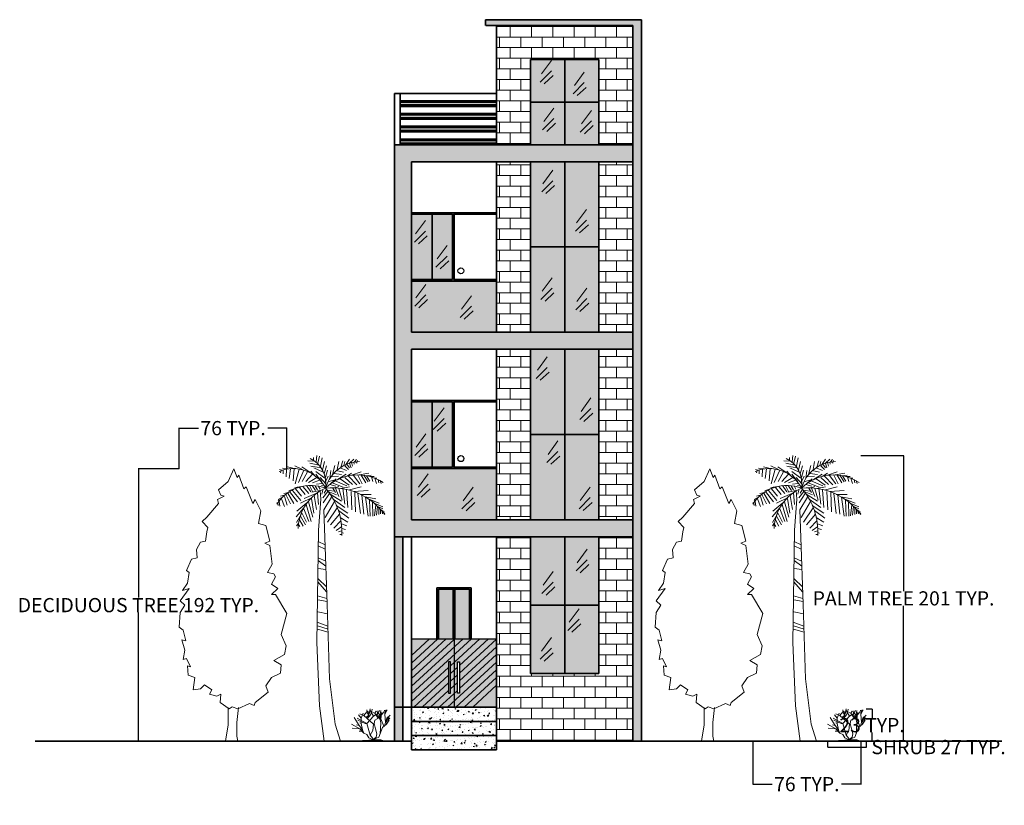
# Model space of a CAD drawing. Units: inches. Extents: x 108 to 802, y 307 to 860.
import ezdxf

# ---------------------------------------------------------------- set-up
doc = ezdxf.new("R2010")
doc.units = ezdxf.units.IN
doc.header["$MEASUREMENT"] = 0
for name, color, linetype, lineweight in [('A-ANNO-DIMS', 2, 'Continuous', 18), ('A-DOOR', 3, 'Continuous', 25), ('A-DOOR-PATT', 18, 'Continuous', 13), ('A-ELEV', 7, 'Continuous', 35), ('A-ELEV-PATT', 251, 'Continuous', 13), ('A-FLOR-STRS', 252, 'Continuous', 13), ('A-GLAZ', 4, 'Continuous', 18), ('A-GLAZ-PATT', 9, 'Continuous', 13), ('A-WALL-PATT', 8, 'Continuous', 13), ('PLANT', 3, 'Continuous', 18)]:
    doc.layers.add(name, color=color, linetype=linetype, lineweight=lineweight)
doc.styles.get("Standard").update_dxf_attribs({"font": 'arial.ttf'})
doc.dimstyles.get("Standard").update_dxf_attribs({"dimtxt": 10, "dimasz": 0.18, "dimexe": 0.18, "dimexo": 0.0625, "dimgap": 0.09, "dimtad": 0, "dimtih": 1, "dimtoh": 1, "dimdec": 0, "dimzin": 0, "dimdsep": 46, "dimlunit": 3, "dimtxsty": 'Standard', "dimcen": 0.09, "dimadec": 0, "dimazin": 0, "dimtfac": 1, "dimtdec": 0, "dimtofl": 0, "dimtmove": 0, "dimatfit": 3, "dimfxl": 1, "dimtolj": 1, "dimtzin": 0, "dimarcsym": 0})

# ---------------------------------------------------------------- blocks, each defined once
blk = doc.blocks.new('Shrub - elevation')
for p, q in [((-12.471, 19.775), (-12.898, 22.044)), ((-11.28, 19.619), (-12.104, 21.184)), ((-11.433, 18.289), (-10.457, 22.749)), ((-8.16, 17.76), (-10.56, 21.6)), ((-9.48, 19.775), (-8.992, 22.592)), ((-7.2, 19.68), (-6.24, 21.12)), ((-5.086, 17.741), (-5.513, 21.34)), ((-5.28, 19.2), (-3.84, 21.6)), ((-3.377, 18.602), (-2.888, 21.575)), ((-0.508, 21.888), (-0.081, 20.558)), ((-0.203, 19.149), (0.102, 21.34)), ((-0.02, 20.01), (0.896, 21.105)), ((0.041, 20.714), (1.384, 22.044)), ((0.102, 21.34), (0.835, 21.888)), ((-18.24, 11.04), (-21.755, 16.655)), ((-12.96, 12.48), (-19.68, 16.32)), ((-13.92, 12.48), (-19.2, 14.88)), ((-16.8, 16.32), (-18.72, 18.72)), ((-14.88, 18.24), (-17.76, 19.2)), ((-16.8, 16.32), (-15.36, 19.68)), ((-16.8, 12.48), (-16.8, 16.32)), ((-14.88, 18.24), (-12.96, 20.64)), ((-8.16, 12), (-14.88, 18.24)), ((-13.325, 16.724), (-11.433, 18.289)), ((-12.96, 12.48), (-8.16, 17.76)), ((-11.677, 19.071), (-12.471, 19.775)), ((-12.043, 15.628), (-11.921, 18.836)), ((-11.982, 16.802), (-10.579, 18.054)), ((-11.921, 18.836), (-10.64, 20.401)), ((-10.579, 18.054), (-9.846, 19.697)), ((-7.2, 19.68), (-8.64, 20.16)), ((-8.16, 17.76), (-5.28, 19.2)), ((-7.68, 12.48), (-7.2, 14.88)), ((-4.8, 16.32), (-7.2, 19.68)), ((-7.2, 14.88), (-3.84, 16.8)), ((-3.377, 15.315), (-5.086, 17.819)), ((-2.88, 12.96), (-4.32, 19.68)), ((-3.84, 16.8), (-0.96, 20.64)), ((-2.766, 16.802), (-3.377, 18.602)), ((-2.88, 15.84), (-2.4, 20.16)), ((-0.96, 10.56), (-2.88, 15.84)), ((0.346, 13.203), (-0.203, 19.149)), ((-0.142, 19.384), (0.59, 20.401)), ((0.346, 13.203), (1.323, 16.254)), ((0.96, 12), (1.44, 15.36)), ((0.96, 12), (2.88, 14.88)), ((1.323, 16.254), (3.642, 18.289)), ((1.44, 15.36), (2.88, 17.28)), ((1.92, 13.44), (2.4, 15.36)), ((2.4, 15.36), (3.36, 16.32)), ((-17.76, 8.64), (-23.663, 11.961)), ((-17.76, 8.64), (-23.128, 9.222)), ((-18.24, 11.04), (-20.16, 11.52)), ((-15.84, 8.16), (-18.24, 11.04)), ((-16.32, 7.2), (-18.24, 7.2)), ((-16.8, 12.48), (-17.76, 12.96)), ((-14.88, 5.76), (-17.76, 8.64)), ((-15.84, 8.16), (-16.8, 12.48)), ((-14.88, 5.76), (-15.84, 8.16)), ((-12.96, 12.48), (-13.92, 12.48)), ((-10.56, 4.32), (-12.96, 12.48)), ((-10.56, 4.32), (-8.64, 7.68)), ((-8.64, 7.68), (-8.16, 12)), ((-6.72, 8.64), (-7.68, 12.48)), ((-5.76, 5.28), (-6.72, 8.64)), ((-4.32, 2.88), (-1.92, 9.6)), ((-3.36, 5.28), (-2.88, 12.96)), ((-1.92, 9.6), (0.96, 12)), ((-0.48, 10.8), (0.346, 13.203)), ((-15.84, 0.48), (-17.76, 0)), ((-13.44, 0.48), (-15.84, 0.48)), ((-12.96, 4.8), (-14.88, 5.76)), ((-9.6, 0.96), (-13.44, 0.48)), ((-11.52, 2.4), (-12.96, 4.8)), ((-9.6, 0.96), (-12.96, 0)), ((-8.64, 0.96), (-11.52, 2.4)), ((-8.64, 1.92), (-10.56, 4.32)), ((-9.6, 0.96), (-7.68, 0.96)), ((-8.64, 0.96), (-4.32, 2.88)), ((-8.64, 0.96), (-6.24, 2.88)), ((-8.64, 0.96), (-8.64, 1.92)), ((-8.64, 0.96), (-2.88, 0.96)), ((-7.68, 0.96), (-6.24, 0.48)), ((-6.24, 2.88), (-5.76, 5.28)), ((-6.24, 0.48), (-3.36, 0)), ((-2.88, 0.96), (0, 0))]:
    blk.add_line(p, q)
blk = doc.blocks.new('Tree - palm elevation')
for p, q in [((-6.727, 197.202), (-11.366, 197.45)), ((-3.441, 194.477), (-10.013, 195.716)), ((-7.5, 199.68), (-7.5, 197.946)), ((-5.567, 196.707), (-4.987, 201.167)), ((-4.407, 195.716), (-3.247, 200.672)), ((-2.474, 193.733), (-1.315, 199.433)), ((-1.121, 190.759), (0.232, 196.955)), ((9.317, 191.255), (10.283, 196.955)), ((11.829, 192.99), (13.182, 197.45)), ((13.956, 194.229), (14.729, 196.955)), ((15.116, 194.477), (17.822, 198.689)), ((16.082, 194.972), (17.822, 192.494)), ((18.015, 195.716), (20.914, 198.689)), ((18.015, 195.468), (18.981, 192.494)), ((19.368, 196.459), (19.948, 193.733)), ((20.914, 196.459), (21.301, 194.972)), ((21.301, 196.459), (22.847, 198.441)), ((22.074, 196.707), (23.427, 195.716)), ((23.234, 196.707), (23.62, 197.698)), ((-29.729, 190.759), (-31.469, 191.255)), ((-30.309, 190.512), (-30.695, 189.025)), ((-25.283, 191.751), (-29.342, 192.246)), ((-28.763, 190.759), (-28.763, 188.281)), ((-26.443, 191.503), (-26.636, 186.051)), ((-20.064, 191.751), (-25.863, 193.238)), ((-23.737, 191.751), (-24.51, 185.06)), ((-21.031, 191.998), (-21.804, 183.325)), ((-15.232, 191.255), (-20.644, 193.981)), ((-17.551, 191.503), (-20.451, 181.343)), ((-14.265, 190.759), (-18.131, 182.086)), ((-9.433, 189.025), (-15.618, 193.238)), ((-11.753, 189.768), (-15.425, 182.83)), ((-8.08, 188.034), (-12.912, 182.83)), ((-1.894, 192.494), (-9.24, 193.733)), ((-6.147, 186.299), (-9.24, 190.264)), ((-0.541, 189.52), (-7.307, 192.494)), ((-5.76, 190.016), (0.618, 185.308)), ((-5.76, 188.034), (-1.508, 182.582)), ((0.038, 188.281), (1.778, 193.981)), ((1.005, 185.803), (2.358, 190.759)), ((4.098, 185.06), (4.678, 190.512)), ((5.837, 187.786), (7.577, 194.229)), ((6.997, 188.529), (12.216, 187.786)), ((8.544, 190.512), (13.763, 189.52)), ((9.51, 184.317), (15.502, 188.034)), ((11.25, 192.494), (15.889, 190.512)), ((14.536, 193.981), (17.242, 191.255)), ((15.695, 186.299), (19.368, 188.777)), ((19.368, 187.29), (26.133, 189.768)), ((24.78, 187.538), (31.546, 188.777)), ((-4.987, 185.803), (-10.979, 182.086)), ((-3.247, 183.821), (-8.08, 181.838)), ((-1.315, 181.591), (-5.374, 181.095)), ((-2.668, 185.803), (1.198, 181.343)), ((1.005, 182.582), (2.938, 186.547)), ((2.938, 182.582), (6.61, 183.821)), ((4.098, 180.847), (8.35, 179.608)), ((4.871, 186.051), (10.09, 186.547)), ((4.871, 181.591), (8.544, 184.812)), ((5.644, 181.838), (13.569, 178.865)), ((7.77, 183.325), (16.082, 179.856)), ((11.25, 184.812), (17.628, 180.352)), ((14.536, 185.803), (19.948, 180.847)), ((17.242, 186.547), (23.041, 180.599)), ((20.721, 187.042), (25.167, 181.343)), ((23.814, 187.29), (26.907, 181.343)), ((26.133, 187.29), (29.419, 181.838)), ((28.066, 187.29), (30.966, 182.582)), ((29.806, 186.795), (32.319, 183.078)), ((29.999, 186.795), (33.092, 187.29)), ((32.512, 186.299), (35.218, 186.299)), ((33.479, 186.051), (34.445, 182.83)), ((35.605, 185.556), (37.151, 185.308)), ((35.798, 185.308), (36.958, 181.591)), ((38.118, 184.317), (38.504, 181.838)), ((39.857, 182.83), (40.244, 181.591)), ((-25.09, 175.148), (-28.376, 174.404)), ((-26.829, 173.661), (-23.544, 167.218)), ((-25.476, 174.652), (-21.224, 167.466)), ((-21.031, 177.626), (-24.897, 176.387)), ((-24.317, 175.891), (-18.711, 168.457)), ((-22.191, 176.635), (-16.391, 169.448)), ((-15.618, 179.36), (-20.644, 178.617)), ((-20.064, 177.626), (-15.812, 172.67)), ((-17.358, 178.617), (-13.299, 173.661)), ((-15.038, 179.36), (-10.786, 174.404)), ((-4.214, 175.148), (-14.072, 170.935)), ((-12.332, 180.104), (-9.433, 175.643)), ((-10.206, 180.104), (-8.08, 175.891)), ((-1.701, 176.882), (-8.66, 175.396)), ((-8.273, 180.104), (-6.147, 176.635)), ((-6.34, 179.608), (-4.6, 177.13)), ((-4.6, 174.9), (-4.021, 166.722)), ((-4.021, 179.36), (-2.861, 177.378)), ((-2.668, 176.387), (-2.376, 170.594)), ((-0.348, 180.352), (-1.894, 180.104)), ((-0.928, 176.882), (-1.508, 173.909)), ((2.551, 175.891), (-0.928, 171.431)), ((3.711, 174.404), (-0.541, 167.961)), ((1.585, 177.13), (0.038, 174.652)), ((1.585, 177.13), (6.61, 176.139)), ((2.938, 175.891), (8.737, 173.413)), ((4.291, 173.909), (12.216, 168.953)), ((6.224, 178.121), (8.157, 175.148)), ((7.384, 178.369), (10.476, 179.36)), ((8.157, 178.121), (10.476, 172.422)), ((10.476, 177.874), (12.796, 169.696)), ((11.829, 177.874), (18.015, 179.113)), ((13.182, 177.874), (14.729, 166.97)), ((15.889, 177.13), (16.855, 164.492)), ((18.015, 177.13), (26.133, 179.113)), ((18.981, 175.891), (19.561, 163.005)), ((20.914, 175.891), (30.966, 176.635)), ((21.688, 175.396), (22.074, 161.518)), ((23.814, 174.404), (25.554, 160.279)), ((25.554, 173.661), (33.285, 173.661)), ((-32.628, 167.961), (-33.208, 167.961)), ((-32.628, 167.713), (-32.435, 165.979)), ((-28.956, 172.174), (-32.435, 170.192)), ((-31.082, 169.944), (-32.435, 169.2)), ((-31.662, 168.705), (-31.082, 165.483)), ((-27.409, 173.413), (-30.695, 172.67)), ((-29.922, 170.687), (-27.989, 165.235)), ((-27.989, 172.422), (-26.056, 166.227)), ((-12.139, 167.961), (-19.098, 162.014)), ((-8.466, 171.678), (-16.585, 167.713)), ((-12.719, 166.722), (-9.046, 154.828)), ((-10.979, 168.457), (-7.887, 157.801)), ((-8.853, 170.935), (-7.113, 160.527)), ((-6.92, 172.917), (-5.374, 163.253)), ((5.257, 171.926), (-0.155, 163.005)), ((7.384, 168.705), (0.812, 157.553)), ((6.417, 170.439), (14.729, 164.492)), ((26.52, 173.165), (28.066, 159.784)), ((28.839, 172.174), (36.378, 170.687)), ((29.226, 171.926), (30.966, 158.545)), ((30.966, 170.687), (38.891, 167.713)), ((32.126, 169.696), (32.512, 158.545)), ((34.058, 168.705), (34.445, 158.545)), ((35.412, 167.713), (41.404, 164.988)), ((-14.265, 164.244), (-19.678, 158.049)), ((-16.005, 160.031), (-19.484, 154.084)), ((-15.618, 160.775), (-12.332, 154.332)), ((-14.265, 163.749), (-10.786, 154.828)), ((9.317, 164.244), (2.358, 154.332)), ((10.863, 159.784), (4.484, 152.35)), ((8.544, 165.979), (16.662, 160.527)), ((10.09, 162.51), (17.435, 157.058)), ((36.378, 166.474), (35.605, 158.792)), ((37.731, 165.235), (36.958, 159.288)), ((37.924, 165.235), (41.404, 163.749)), ((38.504, 164.492), (38.504, 159.536)), ((39.664, 163.253), (42.37, 161.766)), ((39.857, 162.757), (39.857, 160.031)), ((40.824, 161.766), (41.21, 160.031)), ((41.21, 161.518), (42.757, 160.279)), ((-18.131, 153.589), (-19.484, 151.606)), ((-17.358, 155.819), (-14.845, 151.358)), ((-16.585, 158.545), (-13.106, 152.35)), ((11.829, 155.075), (6.804, 150.119)), ((11.443, 157.553), (16.855, 154.332)), ((12.216, 153.093), (16.082, 151.606)), ((-17.938, 152.597), (-16.972, 151.111)), ((12.603, 151.111), (8.544, 148.385)), ((12.216, 148.137), (10.09, 147.393)), ((12.409, 146.898), (13.763, 146.402)), ((12.603, 149.872), (15.116, 149.128)), ((-4.081, 140.645), (0.753, 138.261)), ((12.409, 145.659), (11.056, 145.659)), ((-4.081, 137.547), (0.753, 135.163)), ((-4.081, 129.205), (1.124, 126.821)), ((-4.081, 127.298), (1.31, 123.246)), ((-4.081, 121.578), (1.31, 120.863)), ((-4.453, 112.283), (1.682, 105.133)), ((-4.267, 114.428), (1.682, 108.708)), ((-4.639, 102.273), (1.868, 100.604)), ((-4.453, 99.651), (2.24, 98.459)), ((-4.453, 91.071), (2.426, 89.641)), ((-4.825, 83.921), (2.612, 81.061)), ((-4.639, 81.299), (2.797, 78.916)), ((-4.639, 78.916), (2.797, 76.771))]:
    blk.add_line(p, q)
for points in [[(-2.363, 170.553), (-3.88, 148.505), (-4.988, 69.634), (-3.325, 24.869), (0, 0)], [(-0.116, 162.848), (0.554, 143.532), (2.217, 96.635), (3.88, 44.054), (7.76, 12.079), (11.64, 0)]]:
    blk.add_lwpolyline(points)
for centre, radius, start, end in [((-18.427, 181.448), 19.715, 350.285, 64.11229), ((25.595, 171.567), 25.395, 91.40319, 163.882), ((-21.738, 166.094), 25.899, 27.67115, 112.5305), ((23.687, 155.341), 32.188, 56.19272, 134.3213), ((-9.259, 151.732), 28.386, 68.38311, 147.5322), ((14.394, 148.393), 32.752, 113.7592, 177.4133), ((5.828, 132.718), 45.639, 35.98777, 95.82273), ((-32.8, 147.923), 45.309, 356.1943, 41.37848)]:
    blk.add_arc(centre, radius, start, end)
blk = doc.blocks.new('Tree - type 2 deciduous elevation')
blk.add_lwpolyline([(-2.754, 191.699), (-6.78, 182.851), (-13.682, 176.953), (-11.956, 173.266), (-9.656, 172.529), (-14.257, 170.317), (-13.682, 167.368), (-21.733, 157.783), (-25.184, 154.834), (-21.158, 150.41), (-21.733, 147.461), (-22.884, 140.825), (-26.334, 140.087), (-29.21, 134.926), (-28.635, 129.028), (-32.661, 128.291), (-36.111, 120.18), (-34.386, 118.706), (-35.536, 111.333), (-38.987, 106.171), (-34.386, 107.646), (-40.712, 98.798), (-37.261, 95.849), (-40.712, 90.688), (-41.287, 80.366), (-38.412, 78.154), (-36.686, 70.781), (-39.562, 71.518), (-37.261, 64.145), (-38.412, 57.509), (-36.111, 58.247), (-33.236, 52.348), (-35.536, 53.086), (-34.961, 46.45), (-30.36, 44.975), (-31.51, 36.128), (-26.334, 36.865), (-23.459, 39.814), (-18.283, 36.128), (-20.008, 33.178), (-14.832, 31.704), (-11.956, 33.178), (-12.531, 27.28), (-6.205, 22.856), (-3.905, 24.331), (0.121, 22.856), (8.173, 26.543), (11.624, 25.068), (12.199, 27.28), (21.4, 34.653), (19.675, 39.077), (23.701, 44.975), (30.027, 47.924), (30.602, 53.823), (25.426, 56.772), (32.903, 61.196), (34.053, 67.094), (30.602, 75.205), (34.628, 89.951), (26.576, 103.222), (23.701, 103.222), (28.302, 107.646), (23.701, 110.595), (26.576, 115.756), (25.426, 117.968), (20.825, 118.706), (24.276, 124.604), (22.551, 137.876), (19.1, 139.35), (22.551, 140.825), (19.675, 151.884), (14.499, 153.359), (16.224, 162.207), (12.199, 170.317), (10.473, 167.368), (5.872, 179.165), (4.147, 177.69), (0.696, 187.275), (-0.454, 185.8)], close=True)
for points in [[(-6.813, 23.669), (-6.813, 11.669), (-8.627, 0)], [(0.387, 23.669), (-0.576, 13.271), (-0.576, 3.686), (0, 0)]]:
    blk.add_lwpolyline(points)
blk = doc.blocks.new('*D4')
at = {"layer": 'A-ANNO-DIMS', "color": 0, "lineweight": -2, "transparency": 16777216}
for p, q in [((677.06, 351.62), (677.06, 347.41)), ((677.24, 347.59), (704.19, 347.59)), ((704.37, 351.62), (704.37, 347.41)), ((704.37, 347.59), (704.55, 347.59))]:
    blk.add_line(p, q, dxfattribs=at)
at = {"layer": 'A-ANNO-DIMS', "color": 0, "transparency": 16777216}
for points in [[(677.24, 347.62), (677.24, 347.56), (677.06, 347.59)], [(704.19, 347.62), (704.19, 347.56), (704.37, 347.59)]]:
    blk.add_solid(points, dxfattribs=at)
at = {"layer": 'Defpoints', "color": 0, "transparency": 16777216}
for p in [(677.06, 351.68), (704.37, 351.68), (704.37, 347.59)]:
    blk.add_point(p, dxfattribs=at)
at = {"layer": 'A-ANNO-DIMS', "color": 0, "transparency": 16777216, "insert": (755.34, 347.59), "char_height": 10, "attachment_point": 5}
blk.add_mtext('\\A1;SHRUB 27 TYP.', dxfattribs=at)
blk = doc.blocks.new('*D5')
at = {"layer": 'A-ANNO-DIMS', "color": 0, "lineweight": -2, "transparency": 16777216}
for p, q in [((704.43, 374.43), (708.64, 374.43)), ((708.46, 374.25), (708.46, 368.26)), ((708.46, 351.86), (708.46, 357.86)), ((704.43, 351.68), (708.64, 351.68))]:
    blk.add_line(p, q, dxfattribs=at)
at = {"layer": 'A-ANNO-DIMS', "color": 0, "transparency": 16777216}
for points in [[(708.43, 374.25), (708.49, 374.25), (708.46, 374.43)], [(708.43, 351.86), (708.49, 351.86), (708.46, 351.68)]]:
    blk.add_solid(points, dxfattribs=at)
at = {"layer": 'Defpoints', "color": 0, "transparency": 16777216}
for p in [(704.37, 374.43), (708.46, 374.43), (704.37, 351.68)]:
    blk.add_point(p, dxfattribs=at)
at = {"layer": 'A-ANNO-DIMS', "color": 0, "transparency": 16777216, "insert": (708.46, 363.06), "char_height": 10, "attachment_point": 5}
blk.add_mtext('\\A1;23 TYP.', dxfattribs=at)
blk = doc.blocks.new('*D6')
at = {"layer": 'A-ANNO-DIMS', "color": 0, "lineweight": -2, "transparency": 16777216}
for p, q in [((700.56, 552.85), (730.86, 552.85)), ((730.68, 552.67), (730.68, 457.46)), ((730.68, 351.86), (730.68, 447.07)), ((700.56, 351.68), (730.86, 351.68))]:
    blk.add_line(p, q, dxfattribs=at)
at = {"layer": 'A-ANNO-DIMS', "color": 0, "transparency": 16777216}
for points in [[(730.65, 552.67), (730.71, 552.67), (730.68, 552.85)], [(730.65, 351.86), (730.71, 351.86), (730.68, 351.68)]]:
    blk.add_solid(points, dxfattribs=at)
at = {"layer": 'Defpoints', "color": 0, "transparency": 16777216}
for p in [(700.5, 552.85), (730.68, 552.85), (700.5, 351.68)]:
    blk.add_point(p, dxfattribs=at)
at = {"layer": 'A-ANNO-DIMS', "color": 0, "transparency": 16777216, "insert": (730.68, 452.27), "char_height": 10, "attachment_point": 5}
blk.add_mtext('\\A1;PALM TREE 201 TYP.', dxfattribs=at)
blk = doc.blocks.new('*D7')
at = {"layer": 'A-ANNO-DIMS', "color": 0, "lineweight": -2, "transparency": 16777216}
for p, q in [((624.54, 351.62), (624.54, 321.33)), ((700.5, 351.62), (700.5, 321.33)), ((624.72, 321.51), (638.13, 321.51)), ((700.32, 321.51), (686.91, 321.51))]:
    blk.add_line(p, q, dxfattribs=at)
at = {"layer": 'A-ANNO-DIMS', "color": 0, "transparency": 16777216}
for points in [[(624.72, 321.54), (624.72, 321.48), (624.54, 321.51)], [(700.32, 321.54), (700.32, 321.48), (700.5, 321.51)]]:
    blk.add_solid(points, dxfattribs=at)
at = {"layer": 'Defpoints', "color": 0, "transparency": 16777216}
for p in [(624.54, 351.68), (700.5, 351.68), (700.5, 321.51)]:
    blk.add_point(p, dxfattribs=at)
at = {"layer": 'A-ANNO-DIMS', "color": 0, "transparency": 16777216, "insert": (662.52, 321.51), "char_height": 10, "attachment_point": 5}
blk.add_mtext('\\A1;76 TYP.', dxfattribs=at)
blk = doc.blocks.new('*D8')
at = {"layer": 'A-ANNO-DIMS', "color": 0, "lineweight": -2, "transparency": 16777216}
for p, q in [((220.22, 543.38), (191.35, 543.38)), ((191.53, 543.2), (191.53, 452.8)), ((191.53, 351.86), (191.53, 442.27)), ((220.22, 351.68), (191.35, 351.68))]:
    blk.add_line(p, q, dxfattribs=at)
at = {"layer": 'A-ANNO-DIMS', "color": 0, "transparency": 16777216}
for points in [[(191.5, 543.2), (191.56, 543.2), (191.53, 543.38)], [(191.5, 351.86), (191.56, 351.86), (191.53, 351.68)]]:
    blk.add_solid(points, dxfattribs=at)
at = {"layer": 'Defpoints', "color": 0, "transparency": 16777216}
for p in [(191.53, 543.38), (220.29, 543.38), (220.29, 351.68)]:
    blk.add_point(p, dxfattribs=at)
at = {"layer": 'A-ANNO-DIMS', "color": 0, "transparency": 16777216, "insert": (191.53, 447.53), "char_height": 10, "attachment_point": 5}
blk.add_mtext('\\A1;DECIDUOUS TREE 192 TYP.', dxfattribs=at)
blk = doc.blocks.new('*D9')
at = {"layer": 'A-ANNO-DIMS', "color": 0, "lineweight": -2, "transparency": 16777216}
for p, q in [((220.29, 543.45), (220.29, 572.32)), ((220.47, 572.14), (233.86, 572.14)), ((296.02, 572.14), (282.63, 572.14)), ((296.2, 543.45), (296.2, 572.32))]:
    blk.add_line(p, q, dxfattribs=at)
at = {"layer": 'A-ANNO-DIMS', "color": 0, "transparency": 16777216}
for points in [[(220.47, 572.17), (220.47, 572.11), (220.29, 572.14)], [(296.02, 572.17), (296.02, 572.11), (296.2, 572.14)]]:
    blk.add_solid(points, dxfattribs=at)
at = {"layer": 'Defpoints', "color": 0, "transparency": 16777216}
for p in [(296.2, 572.14), (220.29, 543.38), (296.2, 543.38)]:
    blk.add_point(p, dxfattribs=at)
at = {"layer": 'A-ANNO-DIMS', "color": 0, "transparency": 16777216, "insert": (258.24, 572.14), "char_height": 10, "attachment_point": 5}
blk.add_mtext('\\A1;76 TYP.', dxfattribs=at)

msp = doc.modelspace()

# ---------------------------------------------------------------- hatches: boundary and pattern name
at = {"layer": 'A-DOOR-PATT'}
h = msp.add_hatch(color=256, dxfattribs=at)
h.dxf.hatch_style = 1
h.paths.add_polyline_path([(402.51, 423.68), (396.58, 423.68), (383.92, 412.13), (383.92, 406.72)], flags=17)
h.paths.add_polyline_path([(413.92, 423.27), (413.92, 423.68), (408.44, 423.68), (383.92, 401.3), (383.92, 395.88)])
h.paths.add_polyline_path([(413.92, 412.44), (413.92, 417.86), (383.92, 390.47), (383.92, 385.05)])
h.paths.add_polyline_path([(426.24, 423.68), (420.31, 423.68), (413.92, 417.86), (413.92, 412.44)], flags=17)
h.paths.add_polyline_path([(438.1, 423.68), (432.17, 423.68), (413.92, 407.02), (413.92, 401.61), (416.29, 403.77), (416.29, 407.51), (417.73, 407.51), (417.73, 405.08)])
h.paths.add_polyline_path([(410.12, 403.55), (383.92, 379.63), (383.92, 375.68), (385.53, 375.68), (410.12, 398.14)])
h.paths.add_polyline_path([(443.92, 418.17), (443.92, 423.58), (417.73, 399.66), (417.73, 394.25)])
h.paths.add_polyline_path([(410.12, 387.3), (410.12, 392.72), (391.46, 375.68), (397.4, 375.68)], flags=17)
h.paths.add_polyline_path([(443.92, 407.33), (443.92, 412.75), (417.73, 388.83), (417.73, 385.58), (416.29, 385.58), (416.29, 387.52), (413.92, 385.36), (413.92, 379.94)])
h.paths.add_polyline_path([(413.92, 385.36), (403.33, 375.68), (409.26, 375.68), (413.92, 379.94)])
h.paths.add_polyline_path([(443.92, 396.5), (443.92, 401.92), (415.19, 375.68), (421.13, 375.68)])
h = msp.add_hatch(color=256, dxfattribs=at)
h.dxf.hatch_style = 1
h.paths.add_polyline_path([(413.92, 407.02), (411.55, 404.86), (411.55, 399.44), (413.92, 401.61)])
h.paths.add_polyline_path([(413.92, 390.78), (413.92, 396.19), (411.55, 394.03), (411.55, 388.61)])
h.paths.add_polyline_path([(416.29, 398.36), (413.92, 396.19), (413.92, 390.78), (416.29, 392.94)])
h = msp.add_hatch(color=256, dxfattribs=at)
h.dxf.hatch_style = 1
h.paths.add_polyline_path([(443.92, 391.08), (427.06, 375.68), (443.92, 375.68)])
at = {"layer": 'A-ELEV-PATT'}
h = msp.add_hatch(color=256, dxfattribs=at)
h.dxf.hatch_style = 1
h.paths.add_polyline_path([(443.92, 859.68), (436.15, 859.68), (436.15, 855.68), (443.92, 855.68), (539.92, 855.68), (539.92, 351.68), (545.92, 351.68), (545.92, 859.68)])
h = msp.add_hatch(color=256, dxfattribs=at)
h.dxf.hatch_style = 1
h.paths.add_polyline_path([(443.92, 801.68), (375.92, 801.68), (375.92, 799.68), (443.92, 799.68)])
h.paths.add_polyline_path([(443.92, 792.68), (375.92, 792.68), (375.92, 790.68), (443.92, 790.68)])
h.paths.add_polyline_path([(443.92, 783.68), (375.92, 783.68), (375.92, 781.68), (443.92, 781.68)])
h.paths.add_polyline_path([(443.92, 774.68), (375.92, 774.68), (375.92, 772.68), (443.92, 772.68)])
h = msp.add_hatch(color=256, dxfattribs=at)
h.dxf.hatch_style = 1
h.paths.add_polyline_path([(539.92, 495.68), (539.92, 507.68), (383.92, 507.68), (383.92, 627.68), (539.92, 627.68), (539.92, 639.68), (383.92, 639.68), (383.92, 759.68), (539.92, 759.68), (539.92, 771.68), (371.92, 771.68), (371.92, 495.68)])
h = msp.add_hatch(color=256, dxfattribs=at)
h.dxf.hatch_style = 1
h.paths.add_polyline_path([(371.92, 375.68), (377.92, 375.68), (377.92, 495.68), (371.92, 495.68)])
h = msp.add_hatch(color=256, dxfattribs=at)
h.dxf.hatch_style = 1
h.paths.add_polyline_path([(371.92, 351.68), (377.92, 351.68), (377.92, 375.68), (371.92, 375.68)])
at = {"layer": 'A-FLOR-STRS'}
h = msp.add_hatch(dxfattribs=at)
h.set_pattern_fill('AR-CONC', color=256)
h.set_pattern_definition([(50, (280.963, 0), (7.1726, -0.62752), [0.75, -8.25]), (355, (280.963, 0), (-1.38751, 7.52192), [0.6, -6.6]), (100.4514, (281.5606, -0.052), (5.78509, 6.8944), [0.6374, -7.01142]), (46.1842, (280.963, 2), (10.67241, -1.6552), [1.125, -12.375]), (96.6356, (281.852, 1.862), (9.34662, 9.74119), [0.9561, -10.51714]), (351.1842, (280.963, 2), (9.34662, 9.7412), [0.9, -9.9]), (21, (281.963, 1.5), (5.96907, -4.02619), [0.75, -8.25]), (326, (281.963, 1.5), (2.43315, 7.2515), [0.6, -6.6]), (71.4514, (282.46, 1.1645), (8.40222, 3.22531), [0.6374, -7.01142]), (37.5, (280.963, 0), (0.121599, 3.328939), [0, -6.52, 0, -6.7, 0, -6.625]), (7.5, (280.963, 0), (2.630695, 3.944117), [0, -3.82, 0, -6.37, 0, -2.525]), (327.5, (278.733, 0), (5.338224, -0.225549), [0, -2.5, 0, -7.8, 0, -10.35]), (317.5, (277.733, 0), (5.83186, 1.00105), [0, -3.25, 0, -5.18, 0, -7.35])])
h.paths.add_polyline_path([(443.92, 365.68), (383.92, 365.68), (383.92, 355.68), (443.92, 355.68)])
h.paths.add_polyline_path([(443.92, 351.68), (443.92, 355.68), (383.92, 355.68), (383.92, 351.68), (383.92, 345.68), (443.92, 345.68)])
h.paths.add_polyline_path([(443.92, 375.68), (383.92, 375.68), (383.92, 365.68), (443.92, 365.68)])
at = {"layer": 'A-GLAZ-PATT'}
h = msp.add_hatch(color=256, dxfattribs=at)
h.dxf.hatch_style = 1
h.paths.add_polyline_path([(443.92, 543.68), (383.92, 543.68), (383.92, 507.68), (443.92, 507.68)])
h.paths.add_polyline_path([(412.92, 590.68), (398.42, 590.68), (398.42, 544.68), (412.92, 544.68)])
h.paths.add_polyline_path([(398.42, 590.68), (383.92, 590.68), (383.92, 544.68), (398.42, 544.68)])
h.paths.add_polyline_path([(443.92, 675.68), (383.92, 675.68), (383.92, 639.68), (443.92, 639.68)])
h.paths.add_polyline_path([(412.92, 722.68), (398.42, 722.68), (398.42, 676.68), (412.92, 676.68)])
h.paths.add_polyline_path([(398.42, 722.68), (383.92, 722.68), (383.92, 676.68), (398.42, 676.68)])
h.paths.add_polyline_path([(424.92, 458.68), (414.52, 458.68), (414.52, 423.68), (424.92, 423.68)])
h.paths.add_polyline_path([(413.32, 458.68), (402.92, 458.68), (402.92, 423.68), (413.32, 423.68)])
h.paths.add_polyline_path([(491.92, 801.68), (467.92, 801.68), (467.92, 771.68), (491.92, 771.68)])
h.paths.add_polyline_path([(491.92, 831.68), (467.92, 831.68), (467.92, 801.68), (491.92, 801.68)])
h.paths.add_polyline_path([(515.92, 831.68), (491.92, 831.68), (491.92, 801.68), (515.92, 801.68)])
h.paths.add_polyline_path([(515.92, 801.68), (491.92, 801.68), (491.92, 771.68), (515.92, 771.68)])
h.paths.add_polyline_path([(515.92, 759.68), (491.92, 759.68), (491.92, 699.68), (515.92, 699.68)])
h.paths.add_polyline_path([(491.92, 759.68), (467.92, 759.68), (467.92, 699.68), (491.92, 699.68)])
h.paths.add_polyline_path([(491.92, 699.68), (467.92, 699.68), (467.92, 639.68), (491.92, 639.68)])
h.paths.add_polyline_path([(515.92, 699.68), (491.92, 699.68), (491.92, 639.68), (515.92, 639.68)])
h.paths.add_polyline_path([(491.92, 627.68), (467.92, 627.68), (467.92, 567.68), (491.92, 567.68)])
h.paths.add_polyline_path([(515.92, 627.68), (491.92, 627.68), (491.92, 567.68), (515.92, 567.68)])
h.paths.add_polyline_path([(491.92, 567.68), (467.92, 567.68), (467.92, 507.68), (491.92, 507.68)])
h.paths.add_polyline_path([(515.92, 567.68), (491.92, 567.68), (491.92, 507.68), (515.92, 507.68)])
h.paths.add_polyline_path([(515.92, 495.68), (491.92, 495.68), (491.92, 447.5), (515.92, 447.5)])
h.paths.add_polyline_path([(491.92, 495.68), (467.92, 495.68), (467.92, 447.5), (491.92, 447.5)])
h.paths.add_polyline_path([(491.92, 447.5), (467.92, 447.5), (467.92, 399.32), (491.92, 399.32)])
h.paths.add_polyline_path([(515.92, 447.5), (491.92, 447.5), (491.92, 399.32), (515.92, 399.32)])
h = msp.add_hatch(color=256, dxfattribs=at)
h.dxf.hatch_style = 1
h.paths.add_polyline_path([(410.12, 392.72), (410.12, 398.14), (385.53, 375.68), (391.46, 375.68)])
h.paths.add_polyline_path([(413.92, 401.61), (411.55, 399.44), (411.55, 394.03), (413.92, 396.19)], flags=17)
h.paths.add_polyline_path([(416.29, 403.77), (413.92, 401.61), (413.92, 396.19), (416.29, 398.36)], flags=17)
h.paths.add_polyline_path([(443.92, 423.58), (443.92, 423.68), (438.1, 423.68), (417.73, 405.08), (417.73, 399.66)])
h.paths.add_polyline_path([(443.92, 412.75), (443.92, 418.17), (417.73, 394.25), (417.73, 388.83)])
h.paths.add_polyline_path([(416.29, 392.94), (413.92, 390.78), (413.92, 385.36), (416.29, 387.52)], flags=17)
h.paths.add_polyline_path([(413.92, 390.78), (411.55, 388.61), (411.55, 385.58), (410.12, 385.58), (410.12, 387.3), (397.4, 375.68), (403.33, 375.68), (413.92, 385.36)])
h.paths.add_polyline_path([(443.92, 401.92), (443.92, 407.33), (413.92, 379.94), (413.92, 375.68), (415.19, 375.68)])
h.paths.add_polyline_path([(413.92, 379.94), (409.26, 375.68), (413.92, 375.68)], flags=17)
h.paths.add_polyline_path([(443.92, 391.08), (443.92, 396.5), (421.13, 375.68), (427.06, 375.68)], flags=17)
h.paths.add_polyline_path([(410.12, 403.55), (410.12, 407.51), (411.55, 407.51), (411.55, 404.86), (413.92, 407.02), (413.92, 412.44), (383.92, 385.05), (383.92, 379.63)])
h.paths.add_polyline_path([(432.17, 423.68), (426.24, 423.68), (413.92, 412.44), (413.92, 407.02)])
h.paths.add_polyline_path([(413.92, 417.86), (413.92, 423.27), (383.92, 395.88), (383.92, 390.47)])
h.paths.add_polyline_path([(420.31, 423.68), (413.92, 423.68), (413.92, 417.86)], flags=17)
h.paths.add_polyline_path([(408.44, 423.68), (402.51, 423.68), (383.92, 406.72), (383.92, 401.3)])
h.paths.add_polyline_path([(396.58, 423.68), (383.92, 423.68), (383.92, 412.13)], flags=17)
at = {"layer": 'A-WALL-PATT'}
h = msp.add_hatch(dxfattribs=at)
h.set_pattern_fill('BRICK', color=256, scale=30)
h.set_pattern_definition([(0, (280.963, 0), (0, 7.5), []), (90, (280.963, 0), (-15, 9e-16), [7.5, -7.5]), (90, (288.463, 0), (-15, 9e-16), [-7.5, 7.5])])
h.paths.add_polyline_path([(467.92, 831.68), (515.92, 831.68), (515.92, 771.68), (539.92, 771.68), (539.92, 855.68), (443.92, 855.68), (443.92, 771.68), (467.92, 771.68)])
h.paths.add_polyline_path([(539.92, 759.68), (515.92, 759.68), (515.92, 639.68), (539.92, 639.68)])
h.paths.add_polyline_path([(467.92, 759.68), (443.92, 759.68), (443.92, 639.68), (467.92, 639.68)])
h.paths.add_polyline_path([(467.92, 627.68), (443.92, 627.68), (443.92, 507.68), (467.92, 507.68)])
h.paths.add_polyline_path([(539.92, 627.68), (515.92, 627.68), (515.92, 507.68), (539.92, 507.68)])
h.paths.add_polyline_path([(467.92, 495.68), (443.92, 495.68), (443.92, 375.68), (443.92, 351.68), (539.92, 351.68), (539.92, 495.68), (515.92, 495.68), (515.92, 399.32), (467.92, 399.32)])

# ---------------------------------------------------------------- linework, layer by layer
at = {"layer": 'A-DOOR'}
for p, q in [((383.92, 423.68), (443.92, 423.68)), ((396.58, 423.68), (383.92, 412.13)), ((402.51, 423.68), (383.92, 406.72)), ((408.44, 423.68), (383.92, 401.3)), ((420.31, 423.68), (383.92, 390.47)), ((426.24, 423.68), (383.92, 385.05)), ((413.92, 423.27), (383.92, 395.88)), ((432.17, 423.68), (411.55, 404.86)), ((413.92, 423.68), (413.92, 375.68)), ((438.1, 423.68), (417.73, 405.08)), ((443.92, 423.58), (417.73, 399.66)), ((443.92, 418.17), (417.73, 394.25)), ((443.92, 412.75), (417.73, 388.83)), ((410.12, 403.55), (383.92, 379.63)), ((443.92, 407.33), (409.26, 375.68)), ((416.29, 403.77), (411.55, 399.44)), ((410.12, 398.14), (385.53, 375.68)), ((416.29, 398.36), (411.55, 394.03)), ((443.92, 401.92), (415.19, 375.68)), ((443.92, 396.5), (421.13, 375.68)), ((410.12, 392.72), (391.46, 375.68)), ((416.29, 392.94), (411.55, 388.61)), ((443.92, 391.08), (427.06, 375.68)), ((410.12, 387.3), (397.4, 375.68)), ((416.29, 387.52), (403.33, 375.68))]:
    msp.add_line(p, q, dxfattribs=at)
for points in [[(411.55, 407.51), (410.12, 407.51), (410.12, 385.58), (411.55, 385.58)], [(416.29, 407.51), (417.73, 407.51), (417.73, 385.58), (416.29, 385.58)]]:
    msp.add_lwpolyline(points, close=True, dxfattribs=at)
for centre in [(418.73, 682.88), (418.73, 550.71)]:
    msp.add_circle(centre, 2.13, dxfattribs=at)
at = {"layer": 'A-ELEV'}
for p, q in [((443.92, 859.68), (436.15, 859.68)), ((436.15, 859.68), (436.15, 855.68)), ((443.92, 855.68), (436.28, 855.68)), ((443.92, 859.68), (545.92, 859.68)), ((443.92, 855.68), (443.92, 771.68)), ((443.92, 855.68), (539.92, 855.68)), ((539.92, 855.68), (539.92, 351.68)), ((545.92, 859.68), (545.92, 351.68)), ((467.92, 831.68), (467.92, 771.68)), ((467.92, 831.68), (515.92, 831.68)), ((491.92, 831.68), (491.92, 771.68)), ((515.92, 831.68), (515.92, 771.68)), ((371.92, 807.68), (371.92, 351.68)), ((371.92, 807.68), (443.92, 807.68)), ((375.92, 807.68), (375.92, 771.68)), ((375.92, 802.68), (443.92, 802.68)), ((375.92, 801.68), (443.92, 801.68)), ((375.92, 799.68), (443.92, 799.68)), ((375.92, 798.68), (443.92, 798.68)), ((467.92, 801.68), (515.92, 801.68)), ((375.92, 793.68), (443.92, 793.68)), ((375.92, 792.68), (443.92, 792.68)), ((375.92, 790.68), (443.92, 790.68)), ((375.92, 789.68), (443.92, 789.68)), ((375.92, 784.68), (443.92, 784.68)), ((375.92, 783.68), (443.92, 783.68)), ((375.92, 781.68), (443.92, 781.68)), ((375.92, 780.68), (443.92, 780.68)), ((371.92, 771.68), (539.92, 771.68)), ((375.92, 775.68), (443.92, 775.68)), ((375.92, 774.68), (443.92, 774.68)), ((375.92, 772.68), (443.92, 772.68)), ((383.92, 759.68), (383.92, 639.68)), ((383.92, 759.68), (539.92, 759.68)), ((443.92, 759.68), (443.92, 639.68)), ((467.92, 759.68), (467.92, 639.68)), ((491.92, 759.68), (491.92, 639.68)), ((515.92, 759.68), (515.92, 639.68)), ((383.92, 723.68), (443.92, 723.68)), ((383.92, 722.68), (412.92, 722.68)), ((398.42, 676.68), (398.42, 722.68)), ((412.92, 676.68), (412.92, 722.68)), ((413.92, 675.68), (413.92, 723.68)), ((413.92, 722.68), (443.92, 722.68)), ((467.92, 699.68), (515.92, 699.68)), ((383.92, 676.68), (412.92, 676.68)), ((383.92, 676.68), (412.92, 676.68)), ((383.92, 675.68), (443.92, 675.68)), ((413.92, 676.68), (443.92, 676.68)), ((383.92, 639.68), (539.92, 639.68)), ((383.92, 627.68), (539.92, 627.68)), ((383.92, 627.68), (383.92, 507.68)), ((443.92, 627.68), (443.92, 507.68)), ((467.92, 627.68), (467.92, 507.68)), ((491.92, 627.68), (491.92, 507.68)), ((515.92, 627.68), (515.92, 507.68)), ((383.92, 591.68), (443.92, 591.68)), ((383.92, 590.68), (412.92, 590.68)), ((398.42, 544.68), (398.42, 590.68)), ((412.92, 544.68), (412.92, 590.68)), ((413.92, 543.68), (413.92, 591.68)), ((413.92, 590.68), (443.92, 590.68)), ((467.92, 567.68), (515.92, 567.68)), ((383.92, 544.68), (412.92, 544.68)), ((383.92, 544.68), (412.92, 544.68)), ((383.92, 543.68), (443.92, 543.68)), ((413.92, 544.68), (443.92, 544.68)), ((383.92, 507.68), (539.92, 507.68)), ((371.92, 495.68), (539.92, 495.68)), ((377.92, 495.68), (377.92, 351.68)), ((383.92, 495.68), (383.92, 375.68)), ((443.92, 495.68), (443.92, 375.68)), ((467.92, 495.68), (467.92, 399.32)), ((491.92, 495.68), (491.92, 399.32)), ((515.92, 495.68), (515.92, 399.32)), ((401.92, 423.68), (401.92, 459.68)), ((401.92, 459.68), (425.92, 459.68)), ((402.92, 458.68), (424.92, 458.68)), ((402.92, 423.68), (402.92, 458.68)), ((413.32, 423.68), (413.32, 458.68)), ((414.52, 423.68), (414.52, 458.68)), ((424.92, 423.68), (424.92, 458.68)), ((425.92, 423.68), (425.92, 459.68)), ((467.92, 447.5), (515.92, 447.5)), ((467.92, 399.32), (515.92, 399.32)), ((371.92, 375.68), (443.92, 375.68)), ((383.92, 375.68), (371.92, 375.68)), ((383.92, 375.68), (383.92, 351.68)), ((443.92, 375.68), (443.92, 351.68)), ((383.92, 365.68), (443.92, 365.68)), ((383.92, 355.68), (443.92, 355.68)), ((333.99, 351.68), (118.81, 351.68)), ((371.92, 351.68), (333.99, 351.68)), ((371.92, 351.68), (383.92, 351.68)), ((383.92, 351.68), (383.92, 345.68)), ((443.92, 351.68), (443.92, 345.68)), ((443.92, 351.68), (545.92, 351.68)), ((545.92, 351.68), (610.66, 351.68)), ((610.66, 351.68), (799.8, 351.68)), ((383.92, 345.68), (443.92, 345.68))]:
    msp.add_line(p, q, dxfattribs=at)
at = {"layer": 'A-GLAZ'}
for p, q in [((482.5, 831.08), (475.47, 821.58)), ((482.5, 823.65), (474.65, 815.8)), ((483.74, 820.34), (477.54, 814.57)), ((505.72, 822.79), (498.69, 813.3)), ((505.72, 815.36), (497.87, 807.52)), ((506.96, 812.06), (500.76, 806.28)), ((484.16, 797.52), (477.13, 788.02)), ((510.69, 795.86), (503.67, 786.37)), ((484.16, 790.09), (476.31, 782.24)), ((485.39, 786.78), (479.2, 781.01)), ((510.69, 788.43), (502.84, 780.59)), ((511.93, 785.13), (505.74, 779.35)), ((483.53, 753.72), (476.51, 744.23)), ((483.53, 746.29), (475.68, 738.45)), ((484.77, 742.99), (478.57, 737.21)), ((507.32, 726.08), (500.3, 716.58)), ((393.8, 718.33), (386.78, 708.83)), ((507.32, 718.65), (499.47, 710.8)), ((508.56, 715.34), (502.36, 709.57)), ((393.8, 710.9), (385.95, 703.05)), ((395.04, 707.59), (388.84, 701.81)), ((409.06, 700.75), (402.03, 691.26)), ((409.06, 693.32), (401.21, 685.48)), ((410.3, 690.02), (404.1, 684.24)), ((394.06, 673.37), (387.04, 663.87)), ((483.01, 678.02), (475.99, 668.52)), ((483.01, 670.59), (475.16, 662.74)), ((484.25, 667.28), (478.05, 661.51)), ((507.58, 670.78), (500.56, 661.29)), ((394.06, 665.94), (386.21, 658.09)), ((395.3, 662.63), (389.1, 656.85)), ((426.12, 665.36), (419.1, 655.86)), ((507.58, 663.35), (499.73, 655.51)), ((508.82, 660.05), (502.62, 654.27)), ((426.12, 657.93), (418.27, 650.08)), ((427.36, 654.62), (421.17, 648.84)), ((479.66, 622.34), (472.64, 612.85)), ((479.66, 614.91), (471.81, 607.07)), ((480.9, 611.61), (474.7, 605.83)), ((510.43, 593.4), (503.41, 583.91)), ((407.01, 586.42), (399.99, 576.93)), ((510.43, 585.97), (502.58, 578.13)), ((407.01, 578.99), (399.16, 571.15)), ((511.67, 582.67), (505.47, 576.89)), ((408.25, 575.69), (402.05, 569.91)), ((394.16, 568.19), (387.13, 558.7)), ((487.16, 563.17), (480.14, 553.68)), ((394.16, 560.76), (386.31, 552.92)), ((395.39, 557.46), (389.2, 551.68)), ((487.16, 555.74), (479.31, 547.9)), ((488.4, 552.44), (482.2, 546.66)), ((395.81, 540.02), (388.79, 530.52)), ((395.81, 532.59), (387.97, 524.75)), ((397.05, 529.29), (390.86, 523.51)), ((427.33, 530.49), (420.3, 520.99)), ((509.91, 530.62), (502.89, 521.12)), ((427.33, 523.06), (419.48, 515.22)), ((509.91, 523.19), (502.06, 515.34)), ((428.57, 519.76), (422.37, 513.98)), ((511.15, 519.88), (504.96, 514.1)), ((507.78, 486.84), (500.76, 477.35)), ((507.78, 479.41), (499.93, 471.57)), ((509.02, 476.11), (502.82, 470.33)), ((483.73, 471.1), (476.71, 461.6)), ((483.73, 463.67), (475.88, 455.82)), ((484.97, 460.36), (478.77, 454.59)), ((501.98, 444.99), (494.95, 435.5)), ((501.98, 437.56), (494.13, 429.72)), ((503.22, 434.26), (497.02, 428.48)), ((482.49, 424.69), (475.47, 415.2)), ((482.49, 417.26), (474.64, 409.42)), ((483.73, 413.96), (477.53, 408.18))]:
    msp.add_line(p, q, dxfattribs=at)

# ---------------------------------------------------------------- block references
at = {"layer": 'PLANT'}
for name, p in [('Tree - palm elevation', (322.35, 351.68)), ('Tree - palm elevation', (657.74, 351.68)), ('Tree - type 2 deciduous elevation', (261.57, 351.68)), ('Tree - type 2 deciduous elevation', (596.97, 351.68)), ('Shrub - elevation', (365.33, 351.68)), ('Shrub - elevation', (700.73, 351.68))]:
    msp.add_blockref(name, p, dxfattribs=at)

# ---------------------------------------------------------------- dimensions: what is measured, and where the dimension line sits
at = {"layer": 'A-ANNO-DIMS'}
for base, p1, p2, text, picture, middle in [((296.2, 572.14), (220.29, 543.38), (296.2, 543.38), '<> TYP.', '*D9', (258.24, 572.14)), ((704.37, 347.59), (677.06, 351.68), (704.37, 351.68), 'SHRUB <> TYP.', '*D4', (755.34, 347.59)), ((700.5, 321.51), (624.54, 351.68), (700.5, 351.68), '<> TYP.', '*D7', (662.52, 321.51))]:
    dim = msp.add_linear_dim(base=base, p1=p1, p2=p2, text=text, dimstyle='Standard', override={"dimdec": 0, "dimlfac": 1, "dimrnd": 0, "dimzin": 0, "dimdsep": 46, "dimlunit": 2}, dxfattribs=at)
    dim.commit()
    dim.dimension.update_dxf_attribs({"geometry": picture, "text_midpoint": middle})
for base, p1, p2, text, picture, middle in [((730.68, 552.85), (700.5, 351.68), (700.5, 552.85), 'PALM TREE <> TYP.', '*D6', (730.68, 452.27)), ((191.53, 543.38), (220.29, 351.68), (220.29, 543.38), 'DECIDUOUS TREE <> TYP.', '*D8', (191.53, 447.53)), ((708.46, 374.43), (704.37, 351.68), (704.37, 374.43), '<> TYP.', '*D5', (708.46, 363.06))]:
    dim = msp.add_linear_dim(base=base, p1=p1, p2=p2, angle=90, text=text, dimstyle='Standard', override={"dimdec": 0, "dimlfac": 1, "dimrnd": 0, "dimzin": 0, "dimdsep": 46, "dimlunit": 2}, dxfattribs=at)
    dim.commit()
    dim.dimension.update_dxf_attribs({"geometry": picture, "text_midpoint": middle})

doc.saveas('drawing.dxf')
